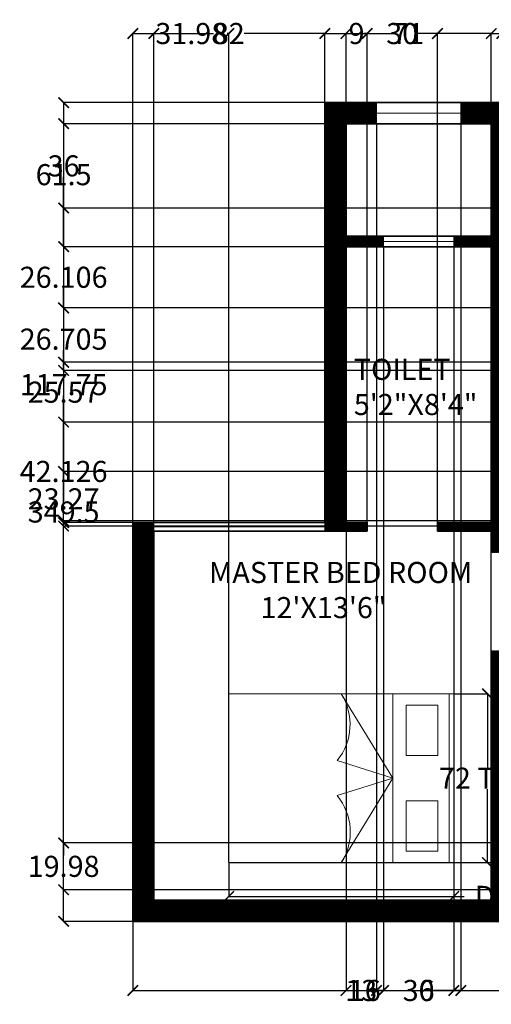
# Model space of a CAD drawing. Units: inches. Extents: x -9 to 675, y 146 to 566.
# Tile 1 of 4: x -9 to 192, y 146 to 566. Entities that reach past the tile are written whole.
import ezdxf

# ---------------------------------------------------------------- set-up
doc = ezdxf.new("R2010")
doc.units = ezdxf.units.IN
doc.header["$MEASUREMENT"] = 0
for name, color, linetype, lineweight in [('A-ANNO-DIMS', 2, 'Continuous', 18), ('A-AREA-IDEN', 7, 'Continuous', 18), ('A-FURN', 8, 'Continuous', 18), ('A-GLAZ', 4, 'Continuous', 18), ('A-WALL', 7, 'Continuous', 35), ('A-WALL-PATT', 252, 'Continuous', 13)]:
    doc.layers.add(name, color=color, linetype=linetype, lineweight=lineweight)
doc.styles.get("Standard").update_dxf_attribs({"font": 'arial.ttf'})
doc.dimstyles.get("Standard").update_dxf_attribs({"dimtxt": 9, "dimasz": 4.5, "dimexe": 0.18, "dimexo": 0.0625, "dimgap": 0.09, "dimtad": 0, "dimtih": 1, "dimtoh": 1, "dimdec": 1, "dimzin": 0, "dimdsep": 46, "dimlunit": 4, "dimtxsty": 'Standard', "dimblk": 'ARCHTICK', "dimcen": 0.09, "dimadec": 0, "dimazin": 0, "dimtfac": 1, "dimtdec": 1, "dimtofl": 0, "dimtmove": 0, "dimatfit": 3, "dimfxl": 1, "dimtolj": 1, "dimtzin": 0, "dimarcsym": 0})

# ---------------------------------------------------------------- blocks, each defined once
blk = doc.blocks.new('BED-DOUBLE-72X96')
for p, q in [((0, 0.1), (0, 72.1)), ((0, 72.1), (96, 72.1)), ((70, 36.1), (48, 72.1)), ((70, 72.1), (70, 0.1)), ((94, 72.1), (94, 0.1)), ((96, 72.1), (96, 0.1)), ((46.29, 43.57), (70, 36.1)), ((70, 36.1), (46.22, 28.65)), ((48, 0.1), (70, 36.1)), ((96, 0.1), (0, 0.1))]:
    blk.add_line(p, q)
for points in [[(89.14, 67.27), (89.14, 45.76), (75.68, 45.76), (75.68, 67.27)], [(89.14, 4.92), (89.14, 26.43), (75.68, 26.43), (75.68, 4.92)]]:
    blk.add_lwpolyline(points, close=True)
for centre, start, end in [((27.13, 59.03), 321.0858, 32.0518), ((27.23, 12.97), 328.2029, 39.5369)]:
    blk.add_arc(centre, 24.62, start, end)
blk = doc.blocks.new('_ArchTick')
at = {"color": 0, "linetype": 'ByBlock', "const_width": 0.15}
blk.add_lwpolyline([(-0.5, -0.5), (0.5, 0.5)], dxfattribs=at)
blk = doc.blocks.new('*D4')
at = {"layer": 'A-ANNO-DIMS', "color": 0, "lineweight": -2, "transparency": 16777216}
for p, q in [((80.28, 206.51), (80.28, 192)), ((176.28, 206.51), (176.28, 192)), ((80.28, 192.18), (176.28, 192.18)), ((176.28, 192.18), (180.78, 192.18))]:
    blk.add_line(p, q, dxfattribs=at)
at = {"layer": 'Defpoints', "color": 0, "transparency": 16777216}
for p in [(80.28, 206.58), (176.28, 206.58), (176.28, 192.18)]:
    blk.add_point(p, dxfattribs=at)
at = {"layer": 'A-ANNO-DIMS', "color": 0, "lineweight": -2, "transparency": 16777216, "xscale": 4.5, "yscale": 4.5, "zscale": 4.5, "rotation": 180}
blk.add_blockref('_ArchTick', (80.28, 192.18), dxfattribs=at)
at = {"layer": 'A-ANNO-DIMS', "color": 0, "lineweight": -2, "transparency": 16777216, "xscale": 4.5, "yscale": 4.5, "zscale": 4.5}
blk.add_blockref('_ArchTick', (176.28, 192.18), dxfattribs=at)
at = {"layer": 'A-ANNO-DIMS', "color": 0, "transparency": 16777216, "insert": (244.83, 192.18), "char_height": 9, "attachment_point": 5}
blk.add_mtext('\\A1;DOUBLE BED 96 TYP.', dxfattribs=at)
blk = doc.blocks.new('*D5')
at = {"layer": 'A-ANNO-DIMS', "color": 0, "lineweight": -2, "transparency": 16777216}
for p, q in [((176.35, 278.67), (190.86, 278.67)), ((190.68, 278.67), (190.68, 247.24)), ((190.68, 206.58), (190.68, 238.01)), ((176.35, 206.58), (190.86, 206.58))]:
    blk.add_line(p, q, dxfattribs=at)
at = {"layer": 'Defpoints', "color": 0, "transparency": 16777216}
for p in [(176.28, 278.67), (190.68, 278.67), (176.28, 206.58)]:
    blk.add_point(p, dxfattribs=at)
at = {"layer": 'A-ANNO-DIMS', "color": 0, "lineweight": -2, "transparency": 16777216, "xscale": 4.5, "yscale": 4.5, "zscale": 4.5}
for p, rotation in [((190.68, 278.67), 90), ((190.68, 206.58), 270)]:
    blk.add_blockref('_ArchTick', p, dxfattribs=dict(at, rotation=rotation))
at = {"layer": 'A-ANNO-DIMS', "color": 0, "transparency": 16777216, "insert": (190.68, 242.63), "char_height": 9, "attachment_point": 5}
blk.add_mtext('\\A1;72 TYP.', dxfattribs=at)
blk = doc.blocks.new('*D8')
at = {"layer": 'A-ANNO-DIMS', "color": 0, "lineweight": -2, "transparency": 16777216}
for p, q in [((626.3, 217.45), (626.3, 151.83)), ((39.3, 181.45), (39.3, 151.83)), ((39.3, 152.01), (322.77, 152.01)), ((626.3, 152.01), (342.83, 152.01))]:
    blk.add_line(p, q, dxfattribs=at)
at = {"layer": 'Defpoints', "color": 0, "transparency": 16777216}
for p in [(626.3, 217.51), (39.3, 181.51), (626.3, 152.01)]:
    blk.add_point(p, dxfattribs=at)
at = {"layer": 'A-ANNO-DIMS', "color": 0, "lineweight": -2, "transparency": 16777216, "xscale": 4.5, "yscale": 4.5, "zscale": 4.5, "rotation": 180}
blk.add_blockref('_ArchTick', (39.3, 152.01), dxfattribs=at)
at = {"layer": 'A-ANNO-DIMS', "color": 0, "lineweight": -2, "transparency": 16777216, "xscale": 4.5, "yscale": 4.5, "zscale": 4.5}
blk.add_blockref('_ArchTick', (626.3, 152.01), dxfattribs=at)
at = {"layer": 'A-ANNO-DIMS', "color": 0, "transparency": 16777216, "insert": (332.8, 152.01), "char_height": 9, "attachment_point": 5}
blk.add_mtext('\\A1;587', dxfattribs=at)
blk = doc.blocks.new('*D9')
at = {"layer": 'A-ANNO-DIMS', "color": 0, "lineweight": -2, "transparency": 16777216}
for p, q in [((121.24, 531.01), (9.62, 531.01)), ((9.8, 531.01), (9.8, 360.95)), ((9.8, 181.51), (9.8, 351.57)), ((39.24, 181.51), (9.62, 181.51))]:
    blk.add_line(p, q, dxfattribs=at)
at = {"layer": 'Defpoints', "color": 0, "transparency": 16777216}
for p in [(9.8, 531.01), (121.3, 531.01), (39.3, 181.51)]:
    blk.add_point(p, dxfattribs=at)
at = {"layer": 'A-ANNO-DIMS', "color": 0, "lineweight": -2, "transparency": 16777216, "xscale": 4.5, "yscale": 4.5, "zscale": 4.5}
for p, rotation in [((9.8, 531.01), 90), ((9.8, 181.51), 270)]:
    blk.add_blockref('_ArchTick', p, dxfattribs=dict(at, rotation=rotation))
at = {"layer": 'A-ANNO-DIMS', "color": 0, "transparency": 16777216, "insert": (9.8, 356.26), "char_height": 9, "attachment_point": 5}
blk.add_mtext('\\A1;349.5', dxfattribs=at)
blk = doc.blocks.new('*D10')
at = {"layer": 'A-ANNO-DIMS', "color": 0, "lineweight": -2, "transparency": 16777216}
for p, q in [((39.3, 351.82), (39.3, 560.69)), ((39.3, 560.51), (73.81, 560.51)), ((121.3, 560.51), (86.8, 560.51)), ((121.3, 351.82), (121.3, 560.69))]:
    blk.add_line(p, q, dxfattribs=at)
at = {"layer": 'Defpoints', "color": 0, "transparency": 16777216}
for p in [(121.3, 560.51), (39.3, 351.76), (121.3, 351.76)]:
    blk.add_point(p, dxfattribs=at)
at = {"layer": 'A-ANNO-DIMS', "color": 0, "lineweight": -2, "transparency": 16777216, "xscale": 4.5, "yscale": 4.5, "zscale": 4.5, "rotation": 180}
blk.add_blockref('_ArchTick', (39.3, 560.51), dxfattribs=at)
at = {"layer": 'A-ANNO-DIMS', "color": 0, "lineweight": -2, "transparency": 16777216, "xscale": 4.5, "yscale": 4.5, "zscale": 4.5}
blk.add_blockref('_ArchTick', (121.3, 560.51), dxfattribs=at)
at = {"layer": 'A-ANNO-DIMS', "color": 0, "transparency": 16777216, "insert": (80.3, 560.51), "char_height": 9, "attachment_point": 5}
blk.add_mtext('\\A1;82', dxfattribs=at)
blk = doc.blocks.new('*D11')
at = {"layer": 'A-ANNO-DIMS', "color": 0, "lineweight": -2, "transparency": 16777216}
for p, q in [((121.3, 531.07), (121.3, 560.69)), ((121.3, 560.51), (151.17, 560.51)), ((192.3, 560.51), (162.43, 560.51)), ((192.3, 522.07), (192.3, 560.69))]:
    blk.add_line(p, q, dxfattribs=at)
at = {"layer": 'Defpoints', "color": 0, "transparency": 16777216}
for p in [(192.3, 560.51), (121.3, 531.01), (192.3, 522.01)]:
    blk.add_point(p, dxfattribs=at)
at = {"layer": 'A-ANNO-DIMS', "color": 0, "lineweight": -2, "transparency": 16777216, "xscale": 4.5, "yscale": 4.5, "zscale": 4.5, "rotation": 180}
blk.add_blockref('_ArchTick', (121.3, 560.51), dxfattribs=at)
at = {"layer": 'A-ANNO-DIMS', "color": 0, "lineweight": -2, "transparency": 16777216, "xscale": 4.5, "yscale": 4.5, "zscale": 4.5}
blk.add_blockref('_ArchTick', (192.3, 560.51), dxfattribs=at)
at = {"layer": 'A-ANNO-DIMS', "color": 0, "transparency": 16777216, "insert": (156.8, 560.51), "char_height": 9, "attachment_point": 5}
blk.add_mtext('\\A1;71', dxfattribs=at)
blk = doc.blocks.new('*D12')
at = {"layer": 'A-ANNO-DIMS', "color": 0, "lineweight": -2, "transparency": 16777216}
for p, q in [((192.3, 522.07), (192.3, 560.69)), ((192.3, 560.51), (227.74, 560.51)), ((286.8, 560.51), (251.37, 560.51)), ((286.8, 531.07), (286.8, 560.69))]:
    blk.add_line(p, q, dxfattribs=at)
at = {"layer": 'Defpoints', "color": 0, "transparency": 16777216}
for p in [(286.8, 560.51), (286.8, 531.01), (192.3, 522.01)]:
    blk.add_point(p, dxfattribs=at)
at = {"layer": 'A-ANNO-DIMS', "color": 0, "lineweight": -2, "transparency": 16777216, "xscale": 4.5, "yscale": 4.5, "zscale": 4.5, "rotation": 180}
blk.add_blockref('_ArchTick', (192.3, 560.51), dxfattribs=at)
at = {"layer": 'A-ANNO-DIMS', "color": 0, "lineweight": -2, "transparency": 16777216, "xscale": 4.5, "yscale": 4.5, "zscale": 4.5}
blk.add_blockref('_ArchTick', (286.8, 560.51), dxfattribs=at)
at = {"layer": 'A-ANNO-DIMS', "color": 0, "transparency": 16777216, "insert": (239.55, 560.51), "char_height": 9, "attachment_point": 5}
blk.add_mtext('\\A1;94.5', dxfattribs=at)
blk = doc.blocks.new('*D16')
at = {"layer": 'A-ANNO-DIMS', "color": 0, "lineweight": -2, "transparency": 16777216}
for p, q in [((130.24, 469.51), (9.62, 469.51)), ((9.8, 469.51), (9.8, 415.32)), ((9.8, 351.76), (9.8, 405.95)), ((121.24, 351.76), (9.62, 351.76))]:
    blk.add_line(p, q, dxfattribs=at)
at = {"layer": 'Defpoints', "color": 0, "transparency": 16777216}
for p in [(9.8, 469.51), (130.3, 469.51), (121.3, 351.76)]:
    blk.add_point(p, dxfattribs=at)
at = {"layer": 'A-ANNO-DIMS', "color": 0, "lineweight": -2, "transparency": 16777216, "xscale": 4.5, "yscale": 4.5, "zscale": 4.5}
for p, rotation in [((9.8, 469.51), 90), ((9.8, 351.76), 270)]:
    blk.add_blockref('_ArchTick', p, dxfattribs=dict(at, rotation=rotation))
at = {"layer": 'A-ANNO-DIMS', "color": 0, "transparency": 16777216, "insert": (9.8, 410.63), "char_height": 9, "attachment_point": 5}
blk.add_mtext('\\A1;117.75', dxfattribs=at)
blk = doc.blocks.new('*D17')
at = {"layer": 'A-ANNO-DIMS', "color": 0, "lineweight": -2, "transparency": 16777216}
for p, q in [((121.24, 531.01), (9.62, 531.01)), ((9.8, 531.01), (9.8, 504.94)), ((9.8, 469.51), (9.8, 495.57)), ((130.24, 469.51), (9.62, 469.51))]:
    blk.add_line(p, q, dxfattribs=at)
at = {"layer": 'Defpoints', "color": 0, "transparency": 16777216}
for p in [(9.8, 531.01), (121.3, 531.01), (130.3, 469.51)]:
    blk.add_point(p, dxfattribs=at)
at = {"layer": 'A-ANNO-DIMS', "color": 0, "lineweight": -2, "transparency": 16777216, "xscale": 4.5, "yscale": 4.5, "zscale": 4.5}
for p, rotation in [((9.8, 531.01), 90), ((9.8, 469.51), 270)]:
    blk.add_blockref('_ArchTick', p, dxfattribs=dict(at, rotation=rotation))
at = {"layer": 'A-ANNO-DIMS', "color": 0, "transparency": 16777216, "insert": (9.8, 500.26), "char_height": 9, "attachment_point": 5}
blk.add_mtext('\\A1;61.5', dxfattribs=at)
blk = doc.blocks.new('*D24')
at = {"layer": 'A-ANNO-DIMS', "color": 0, "lineweight": -2, "transparency": 16777216}
for p, q in [((130.3, 521.95), (130.3, 151.83)), ((143.3, 521.95), (143.3, 151.83)), ((130.3, 152.01), (130.69, 152.01)), ((143.3, 152.01), (142.92, 152.01))]:
    blk.add_line(p, q, dxfattribs=at)
at = {"layer": 'Defpoints', "color": 0, "transparency": 16777216}
for p in [(130.3, 522.01), (143.3, 522.01), (143.3, 152.01)]:
    blk.add_point(p, dxfattribs=at)
at = {"layer": 'A-ANNO-DIMS', "color": 0, "lineweight": -2, "transparency": 16777216, "xscale": 4.5, "yscale": 4.5, "zscale": 4.5, "rotation": 180}
blk.add_blockref('_ArchTick', (130.3, 152.01), dxfattribs=at)
at = {"layer": 'A-ANNO-DIMS', "color": 0, "lineweight": -2, "transparency": 16777216, "xscale": 4.5, "yscale": 4.5, "zscale": 4.5}
blk.add_blockref('_ArchTick', (143.3, 152.01), dxfattribs=at)
at = {"layer": 'A-ANNO-DIMS', "color": 0, "transparency": 16777216, "insert": (136.8, 152.01), "char_height": 9, "attachment_point": 5}
blk.add_mtext('\\A1;13', dxfattribs=at)
blk = doc.blocks.new('*D25')
at = {"layer": 'A-ANNO-DIMS', "color": 0, "lineweight": -2, "transparency": 16777216}
for p, q in [((143.3, 521.95), (143.3, 151.83)), ((179.3, 521.95), (179.3, 151.83)), ((143.3, 152.01), (154.77, 152.01)), ((179.3, 152.01), (167.83, 152.01))]:
    blk.add_line(p, q, dxfattribs=at)
at = {"layer": 'Defpoints', "color": 0, "transparency": 16777216}
for p in [(143.3, 522.01), (179.3, 522.01), (179.3, 152.01)]:
    blk.add_point(p, dxfattribs=at)
at = {"layer": 'A-ANNO-DIMS', "color": 0, "lineweight": -2, "transparency": 16777216, "xscale": 4.5, "yscale": 4.5, "zscale": 4.5, "rotation": 180}
blk.add_blockref('_ArchTick', (143.3, 152.01), dxfattribs=at)
at = {"layer": 'A-ANNO-DIMS', "color": 0, "lineweight": -2, "transparency": 16777216, "xscale": 4.5, "yscale": 4.5, "zscale": 4.5}
blk.add_blockref('_ArchTick', (179.3, 152.01), dxfattribs=at)
at = {"layer": 'A-ANNO-DIMS', "color": 0, "transparency": 16777216, "insert": (161.3, 152.01), "char_height": 9, "attachment_point": 5}
blk.add_mtext('\\A1;36', dxfattribs=at)
blk = doc.blocks.new('*D31')
at = {"layer": 'A-ANNO-DIMS', "color": 0, "lineweight": -2, "transparency": 16777216}
for p, q in [((130.3, 351.82), (130.3, 560.69)), ((130.3, 560.51), (131.75, 560.51)), ((139.3, 560.51), (137.85, 560.51)), ((139.3, 351.82), (139.3, 560.69))]:
    blk.add_line(p, q, dxfattribs=at)
at = {"layer": 'Defpoints', "color": 0, "transparency": 16777216}
for p in [(139.3, 560.51), (130.3, 351.76), (139.3, 351.76)]:
    blk.add_point(p, dxfattribs=at)
at = {"layer": 'A-ANNO-DIMS', "color": 0, "lineweight": -2, "transparency": 16777216, "xscale": 4.5, "yscale": 4.5, "zscale": 4.5, "rotation": 180}
blk.add_blockref('_ArchTick', (130.3, 560.51), dxfattribs=at)
at = {"layer": 'A-ANNO-DIMS', "color": 0, "lineweight": -2, "transparency": 16777216, "xscale": 4.5, "yscale": 4.5, "zscale": 4.5}
blk.add_blockref('_ArchTick', (139.3, 560.51), dxfattribs=at)
at = {"layer": 'A-ANNO-DIMS', "color": 0, "transparency": 16777216, "insert": (134.8, 560.51), "char_height": 9, "attachment_point": 5}
blk.add_mtext('\\A1;9', dxfattribs=at)
blk = doc.blocks.new('*D32')
at = {"layer": 'A-ANNO-DIMS', "color": 0, "lineweight": -2, "transparency": 16777216}
for p, q in [((139.3, 351.82), (139.3, 560.69)), ((139.3, 560.51), (147.78, 560.51)), ((169.3, 560.51), (160.82, 560.51)), ((169.3, 351.82), (169.3, 560.69))]:
    blk.add_line(p, q, dxfattribs=at)
at = {"layer": 'Defpoints', "color": 0, "transparency": 16777216}
for p in [(169.3, 560.51), (139.3, 351.76), (169.3, 351.76)]:
    blk.add_point(p, dxfattribs=at)
at = {"layer": 'A-ANNO-DIMS', "color": 0, "lineweight": -2, "transparency": 16777216, "xscale": 4.5, "yscale": 4.5, "zscale": 4.5, "rotation": 180}
blk.add_blockref('_ArchTick', (139.3, 560.51), dxfattribs=at)
at = {"layer": 'A-ANNO-DIMS', "color": 0, "lineweight": -2, "transparency": 16777216, "xscale": 4.5, "yscale": 4.5, "zscale": 4.5}
blk.add_blockref('_ArchTick', (169.3, 560.51), dxfattribs=at)
at = {"layer": 'A-ANNO-DIMS', "color": 0, "transparency": 16777216, "insert": (154.3, 560.51), "char_height": 9, "attachment_point": 5}
blk.add_mtext('\\A1;30', dxfattribs=at)
blk = doc.blocks.new('*D39')
at = {"layer": 'A-ANNO-DIMS', "color": 0, "lineweight": -2, "transparency": 16777216}
for p, q in [((357.24, 214.99), (9.62, 214.99)), ((9.8, 214.99), (9.8, 209.69)), ((9.8, 195.01), (9.8, 200.32)), ((357.24, 195.01), (9.62, 195.01))]:
    blk.add_line(p, q, dxfattribs=at)
at = {"layer": 'Defpoints', "color": 0, "transparency": 16777216}
for p in [(9.8, 214.99), (357.3, 214.99), (357.3, 195.01)]:
    blk.add_point(p, dxfattribs=at)
at = {"layer": 'A-ANNO-DIMS', "color": 0, "lineweight": -2, "transparency": 16777216, "xscale": 4.5, "yscale": 4.5, "zscale": 4.5}
for p, rotation in [((9.8, 214.99), 90), ((9.8, 195.01), 270)]:
    blk.add_blockref('_ArchTick', p, dxfattribs=dict(at, rotation=rotation))
at = {"layer": 'A-ANNO-DIMS', "color": 0, "transparency": 16777216, "insert": (9.8, 205), "char_height": 9, "attachment_point": 5}
blk.add_mtext('\\A1;19.98', dxfattribs=at)
blk = doc.blocks.new('*D40')
at = {"layer": 'A-ANNO-DIMS', "color": 0, "lineweight": -2, "transparency": 16777216}
for p, q in [((146.3, 469.45), (146.3, 151.83)), ((176.3, 469.45), (176.3, 151.83)), ((146.3, 152.01), (154.78, 152.01)), ((176.3, 152.01), (167.82, 152.01))]:
    blk.add_line(p, q, dxfattribs=at)
at = {"layer": 'Defpoints', "color": 0, "transparency": 16777216}
for p in [(146.3, 469.51), (176.3, 469.51), (176.3, 152.01)]:
    blk.add_point(p, dxfattribs=at)
at = {"layer": 'A-ANNO-DIMS', "color": 0, "lineweight": -2, "transparency": 16777216, "xscale": 4.5, "yscale": 4.5, "zscale": 4.5, "rotation": 180}
blk.add_blockref('_ArchTick', (146.3, 152.01), dxfattribs=at)
at = {"layer": 'A-ANNO-DIMS', "color": 0, "lineweight": -2, "transparency": 16777216, "xscale": 4.5, "yscale": 4.5, "zscale": 4.5}
blk.add_blockref('_ArchTick', (176.3, 152.01), dxfattribs=at)
at = {"layer": 'A-ANNO-DIMS', "color": 0, "transparency": 16777216, "insert": (161.3, 152.01), "char_height": 9, "attachment_point": 5}
blk.add_mtext('\\A1;30', dxfattribs=at)
blk = doc.blocks.new('*D41')
at = {"layer": 'A-ANNO-DIMS', "color": 0, "lineweight": -2, "transparency": 16777216}
for p, q in [((130.3, 469.45), (130.3, 151.83)), ((146.3, 469.45), (146.3, 151.83)), ((130.3, 152.01), (132.19, 152.01)), ((146.3, 152.01), (144.41, 152.01))]:
    blk.add_line(p, q, dxfattribs=at)
at = {"layer": 'Defpoints', "color": 0, "transparency": 16777216}
for p in [(130.3, 469.51), (146.3, 469.51), (146.3, 152.01)]:
    blk.add_point(p, dxfattribs=at)
at = {"layer": 'A-ANNO-DIMS', "color": 0, "lineweight": -2, "transparency": 16777216, "xscale": 4.5, "yscale": 4.5, "zscale": 4.5, "rotation": 180}
blk.add_blockref('_ArchTick', (130.3, 152.01), dxfattribs=at)
at = {"layer": 'A-ANNO-DIMS', "color": 0, "lineweight": -2, "transparency": 16777216, "xscale": 4.5, "yscale": 4.5, "zscale": 4.5}
blk.add_blockref('_ArchTick', (146.3, 152.01), dxfattribs=at)
at = {"layer": 'A-ANNO-DIMS', "color": 0, "transparency": 16777216, "insert": (138.3, 152.01), "char_height": 9, "attachment_point": 5}
blk.add_mtext('\\A1;16', dxfattribs=at)
blk = doc.blocks.new('*D44')
at = {"layer": 'A-ANNO-DIMS', "color": 0, "lineweight": -2, "transparency": 16777216}
for p, q in [((48.3, 190.57), (48.3, 560.69)), ((48.3, 560.51), (49.01, 560.51)), ((80.28, 560.51), (79.57, 560.51)), ((80.28, 206.74), (80.28, 560.69))]:
    blk.add_line(p, q, dxfattribs=at)
at = {"layer": 'Defpoints', "color": 0, "transparency": 16777216}
for p in [(80.28, 560.51), (80.28, 206.67), (48.3, 190.51)]:
    blk.add_point(p, dxfattribs=at)
at = {"layer": 'A-ANNO-DIMS', "color": 0, "lineweight": -2, "transparency": 16777216, "xscale": 4.5, "yscale": 4.5, "zscale": 4.5, "rotation": 180}
blk.add_blockref('_ArchTick', (48.3, 560.51), dxfattribs=at)
at = {"layer": 'A-ANNO-DIMS', "color": 0, "lineweight": -2, "transparency": 16777216, "xscale": 4.5, "yscale": 4.5, "zscale": 4.5}
blk.add_blockref('_ArchTick', (80.28, 560.51), dxfattribs=at)
at = {"layer": 'A-ANNO-DIMS', "color": 0, "transparency": 16777216, "insert": (64.29, 560.51), "char_height": 9, "attachment_point": 5}
blk.add_mtext('\\A1;31.98', dxfattribs=at)
blk = doc.blocks.new('*D45')
at = {"layer": 'A-ANNO-DIMS', "color": 0, "lineweight": -2, "transparency": 16777216}
for p, q in [((80.35, 206.67), (655.98, 206.67)), ((655.8, 206.67), (655.8, 203.28)), ((655.8, 190.51), (655.8, 193.91)), ((48.37, 190.51), (655.98, 190.51))]:
    blk.add_line(p, q, dxfattribs=at)
at = {"layer": 'Defpoints', "color": 0, "transparency": 16777216}
for p in [(80.28, 206.67), (655.8, 206.67), (48.3, 190.51)]:
    blk.add_point(p, dxfattribs=at)
at = {"layer": 'A-ANNO-DIMS', "color": 0, "lineweight": -2, "transparency": 16777216, "xscale": 4.5, "yscale": 4.5, "zscale": 4.5}
for p, rotation in [((655.8, 206.67), 90), ((655.8, 190.51), 270)]:
    blk.add_blockref('_ArchTick', p, dxfattribs=dict(at, rotation=rotation))
at = {"layer": 'A-ANNO-DIMS', "color": 0, "transparency": 16777216, "insert": (655.8, 198.59), "char_height": 9, "attachment_point": 5}
blk.add_mtext('\\A1;16.165', dxfattribs=at)
blk = doc.blocks.new('*D46')
at = {"layer": 'A-ANNO-DIMS', "color": 0, "lineweight": -2, "transparency": 16777216}
for p, q in [((435.74, 522.01), (9.62, 522.01)), ((9.8, 522.01), (9.8, 508.7)), ((9.8, 486.01), (9.8, 499.32)), ((445.74, 486.01), (9.62, 486.01))]:
    blk.add_line(p, q, dxfattribs=at)
at = {"layer": 'Defpoints', "color": 0, "transparency": 16777216}
for p in [(435.8, 522.01), (9.8, 486.01), (445.8, 486.01)]:
    blk.add_point(p, dxfattribs=at)
at = {"layer": 'A-ANNO-DIMS', "color": 0, "lineweight": -2, "transparency": 16777216, "xscale": 4.5, "yscale": 4.5, "zscale": 4.5}
for p, rotation in [((9.8, 522.01), 90), ((9.8, 486.01), 270)]:
    blk.add_blockref('_ArchTick', p, dxfattribs=dict(at, rotation=rotation))
at = {"layer": 'A-ANNO-DIMS', "color": 0, "transparency": 16777216, "insert": (9.8, 504.01), "char_height": 9, "attachment_point": 5}
blk.add_mtext('\\A1;36', dxfattribs=at)
blk = doc.blocks.new('*D47')
at = {"layer": 'A-ANNO-DIMS', "color": 0, "lineweight": -2, "transparency": 16777216}
for p, q in [((617.24, 373.51), (9.62, 373.51)), ((9.8, 373.51), (9.8, 366.56)), ((9.8, 350.24), (9.8, 357.19)), ((602.52, 350.24), (9.62, 350.24))]:
    blk.add_line(p, q, dxfattribs=at)
at = {"layer": 'Defpoints', "color": 0, "transparency": 16777216}
for p in [(617.3, 373.51), (9.8, 350.24), (602.59, 350.24)]:
    blk.add_point(p, dxfattribs=at)
at = {"layer": 'A-ANNO-DIMS', "color": 0, "lineweight": -2, "transparency": 16777216, "xscale": 4.5, "yscale": 4.5, "zscale": 4.5}
for p, rotation in [((9.8, 373.51), 90), ((9.8, 350.24), 270)]:
    blk.add_blockref('_ArchTick', p, dxfattribs=dict(at, rotation=rotation))
at = {"layer": 'A-ANNO-DIMS', "color": 0, "transparency": 16777216, "insert": (9.8, 361.87), "char_height": 9, "attachment_point": 5}
blk.add_mtext('\\A1;23.27', dxfattribs=at)
blk = doc.blocks.new('*D50')
at = {"layer": 'A-ANNO-DIMS', "color": 0, "lineweight": -2, "transparency": 16777216}
for p, q in [((192.3, 297.07), (192.3, 560.69)), ((192.3, 560.51), (196.8, 560.51)), ((196.8, 297.07), (196.8, 560.69)), ((196.8, 560.51), (201.3, 560.51))]:
    blk.add_line(p, q, dxfattribs=at)
at = {"layer": 'Defpoints', "color": 0, "transparency": 16777216}
for p in [(196.8, 560.51), (192.3, 297.01), (196.8, 297.01)]:
    blk.add_point(p, dxfattribs=at)
at = {"layer": 'A-ANNO-DIMS', "color": 0, "lineweight": -2, "transparency": 16777216, "xscale": 4.5, "yscale": 4.5, "zscale": 4.5, "rotation": 180}
blk.add_blockref('_ArchTick', (192.3, 560.51), dxfattribs=at)
at = {"layer": 'A-ANNO-DIMS', "color": 0, "lineweight": -2, "transparency": 16777216, "xscale": 4.5, "yscale": 4.5, "zscale": 4.5}
blk.add_blockref('_ArchTick', (196.8, 560.51), dxfattribs=at)
at = {"layer": 'A-ANNO-DIMS', "color": 0, "transparency": 16777216, "insert": (209.8, 560.51), "char_height": 9, "attachment_point": 5}
blk.add_mtext('\\A1;4.5', dxfattribs=at)
blk = doc.blocks.new('*D52')
at = {"layer": 'A-ANNO-DIMS', "color": 0, "lineweight": -2, "transparency": 16777216}
for p, q in [((266.3, 443.4), (9.62, 443.4)), ((9.8, 443.4), (9.8, 434.74)), ((9.8, 416.7), (9.8, 425.37)), ((266.3, 416.7), (9.62, 416.7))]:
    blk.add_line(p, q, dxfattribs=at)
at = {"layer": 'Defpoints', "color": 0, "transparency": 16777216}
for p in [(9.8, 443.4), (266.36, 443.4), (266.36, 416.7)]:
    blk.add_point(p, dxfattribs=at)
at = {"layer": 'A-ANNO-DIMS', "color": 0, "lineweight": -2, "transparency": 16777216, "xscale": 4.5, "yscale": 4.5, "zscale": 4.5}
for p, rotation in [((9.8, 443.4), 90), ((9.8, 416.7), 270)]:
    blk.add_blockref('_ArchTick', p, dxfattribs=dict(at, rotation=rotation))
at = {"layer": 'A-ANNO-DIMS', "color": 0, "transparency": 16777216, "insert": (9.8, 430.05), "char_height": 9, "attachment_point": 5}
blk.add_mtext('\\A1;26.705', dxfattribs=at)
blk = doc.blocks.new('*D53')
at = {"layer": 'A-ANNO-DIMS', "color": 0, "lineweight": -2, "transparency": 16777216}
for p, q in [((261.31, 469.51), (9.62, 469.51)), ((9.8, 469.51), (9.8, 461.14)), ((9.8, 443.4), (9.8, 451.77)), ((266.3, 443.4), (9.62, 443.4))]:
    blk.add_line(p, q, dxfattribs=at)
at = {"layer": 'Defpoints', "color": 0, "transparency": 16777216}
for p in [(261.37, 469.51), (9.8, 443.4), (266.36, 443.4)]:
    blk.add_point(p, dxfattribs=at)
at = {"layer": 'A-ANNO-DIMS', "color": 0, "lineweight": -2, "transparency": 16777216, "xscale": 4.5, "yscale": 4.5, "zscale": 4.5}
for p, rotation in [((9.8, 469.51), 90), ((9.8, 443.4), 270)]:
    blk.add_blockref('_ArchTick', p, dxfattribs=dict(at, rotation=rotation))
at = {"layer": 'A-ANNO-DIMS', "color": 0, "transparency": 16777216, "insert": (9.8, 456.46), "char_height": 9, "attachment_point": 5}
blk.add_mtext('\\A1;26.106', dxfattribs=at)
blk = doc.blocks.new('*D55')
at = {"layer": 'A-ANNO-DIMS', "color": 0, "lineweight": -2, "transparency": 16777216}
for p, q in [((202.15, 420.2), (9.62, 420.2)), ((9.8, 420.2), (9.8, 412.11)), ((9.8, 394.64), (9.8, 402.74)), ((202.15, 394.64), (9.62, 394.64))]:
    blk.add_line(p, q, dxfattribs=at)
at = {"layer": 'Defpoints', "color": 0, "transparency": 16777216}
for p in [(9.8, 420.2), (202.21, 420.2), (202.21, 394.64)]:
    blk.add_point(p, dxfattribs=at)
at = {"layer": 'A-ANNO-DIMS', "color": 0, "lineweight": -2, "transparency": 16777216, "xscale": 4.5, "yscale": 4.5, "zscale": 4.5}
for p, rotation in [((9.8, 420.2), 90), ((9.8, 394.64), 270)]:
    blk.add_blockref('_ArchTick', p, dxfattribs=dict(at, rotation=rotation))
at = {"layer": 'A-ANNO-DIMS', "color": 0, "transparency": 16777216, "insert": (9.8, 407.42), "char_height": 9, "attachment_point": 5}
blk.add_mtext('\\A1;25.57', dxfattribs=at)
blk = doc.blocks.new('*D56')
at = {"layer": 'A-ANNO-DIMS', "color": 0, "lineweight": -2, "transparency": 16777216}
for p, q in [((202.15, 394.64), (9.62, 394.64)), ((9.8, 394.64), (9.8, 378.26)), ((9.8, 352.51), (9.8, 368.89)), ((196.74, 352.51), (9.62, 352.51))]:
    blk.add_line(p, q, dxfattribs=at)
at = {"layer": 'Defpoints', "color": 0, "transparency": 16777216}
for p in [(9.8, 394.64), (202.21, 394.64), (196.8, 352.51)]:
    blk.add_point(p, dxfattribs=at)
at = {"layer": 'A-ANNO-DIMS', "color": 0, "lineweight": -2, "transparency": 16777216, "xscale": 4.5, "yscale": 4.5, "zscale": 4.5}
for p, rotation in [((9.8, 394.64), 90), ((9.8, 352.51), 270)]:
    blk.add_blockref('_ArchTick', p, dxfattribs=dict(at, rotation=rotation))
at = {"layer": 'A-ANNO-DIMS', "color": 0, "transparency": 16777216, "insert": (9.8, 373.57), "char_height": 9, "attachment_point": 5}
blk.add_mtext('\\A1;42.126', dxfattribs=at)

msp = doc.modelspace()

# ---------------------------------------------------------------- hatches: boundary and pattern name
at = {"layer": 'A-WALL-PATT'}
h = msp.add_hatch(dxfattribs=at)
h.set_pattern_fill('ANSI31', color=256)
h.paths.add_polyline_path([(361.8026, 244.5097), (357.3026, 244.5097), (357.3026, 228.4917), (286.8026, 228.4917), (196.8026, 228.4917), (196.8026, 297.0097), (192.3026, 297.0097), (192.3026, 190.5097), (196.8026, 190.5097), (196.8026, 219.4917), (286.8026, 219.4917), (357.3026, 219.4917), (357.3026, 217.5097), (357.3026, 214.9917), (361.8026, 214.9917), (361.8026, 217.5097)])
h.paths.add_polyline_path([(532.6092, 217.5097), (541.8026, 217.5097), (550.8026, 217.5097), (626.3026, 217.5097), (626.3026, 373.5097), (626.3026, 378.0097), (617.3026, 378.0097), (617.3026, 373.5097), (617.3026, 226.5097), (550.8026, 226.5097), (541.8026, 226.5097), (488.3026, 226.5097), (488.3026, 331.0097), (483.8026, 331.0097), (474.8026, 331.0097), (474.8026, 326.5097), (483.8026, 326.5097), (483.8026, 226.5097), (421.8026, 226.5097), (421.8026, 326.5097), (444.8026, 326.5097), (444.8026, 331.0097), (421.8026, 331.0097), (417.3026, 331.0097), (417.3026, 217.5097), (417.3026, 190.5097), (387.6027, 190.5097), (361.8026, 190.5097), (361.8026, 195.0097), (357.3026, 195.0097), (357.3026, 190.5097), (357.3026, 181.5097), (387.6027, 181.5097), (421.8026, 181.5097), (532.6092, 181.5097)])
h.paths.add_polyline_path([(421.8026, 190.5097), (421.8026, 217.5097), (523.6092, 217.5097), (523.6092, 190.5097)], flags=16)
h.paths.add_polyline_path([(550.8026, 378.0097), (550.8026, 531.0097), (525.3955, 531.0097), (525.3955, 522.0097), (541.8026, 522.0097), (541.8026, 378.0097), (472.8026, 378.0097), (472.8026, 373.5097), (483.8026, 373.5097), (488.3026, 373.5097), (541.8026, 373.5097), (550.8026, 373.5097)])
h.paths.add_polyline_path([(130.3026, 469.5097), (146.3026, 469.5097), (146.3026, 474.0097), (130.3026, 474.0097), (130.3026, 522.0097), (143.3026, 522.0097), (143.3026, 531.0097), (121.3026, 531.0097), (121.3026, 351.7597), (121.3026, 348.0097), (130.3026, 348.0097), (139.3026, 348.0097), (139.3026, 351.7597), (130.3026, 351.7597)])
h.paths.add_polyline_path([(211.9624, 531.0097), (179.3026, 531.0097), (179.3026, 522.0097), (192.3026, 522.0097), (192.3026, 474.0097), (176.3026, 474.0097), (176.3026, 469.5097), (192.3026, 469.5097), (192.3026, 351.7597), (169.3026, 351.7597), (169.3026, 348.0097), (192.3026, 348.0097), (192.3026, 339.0097), (196.8026, 339.0097), (196.8026, 348.0097), (226.8026, 348.0097), (226.8026, 352.5097), (196.8026, 352.5097), (196.8026, 469.5097), (226.8026, 469.5097), (226.8026, 474.0097), (196.8026, 474.0097), (196.8026, 522.0097), (211.9624, 522.0097)])
h.paths.add_polyline_path([(291.3026, 522.0097), (291.3026, 531.0097), (286.8026, 531.0097), (286.8026, 522.0097), (286.8026, 352.5097), (256.8026, 352.5097), (256.8026, 348.0097), (286.8026, 348.0097), (286.8026, 346.5097), (291.3026, 346.5097)])
h.paths.add_polyline_path([(417.3026, 474.0097), (291.3026, 474.0097), (291.3026, 469.5097), (417.3026, 469.5097)])
h.paths.add_polyline_path([(421.8026, 522.0097), (435.8002, 522.0097), (435.8002, 531.0097), (417.3026, 531.0097), (417.3026, 522.0097), (417.3026, 373.5097), (421.8026, 373.5097), (430.8026, 373.5097), (430.8026, 378.0097), (421.8026, 378.0097)])
h.paths.add_polyline_path([(48.3026, 348.0097), (48.3026, 351.7597), (39.3026, 351.7597), (39.3026, 348.0097), (39.3026, 181.5097), (121.3026, 181.5097), (196.8026, 181.5097), (196.8026, 190.5097), (192.3026, 190.5097), (121.3026, 190.5097), (48.3026, 190.5097)])

# ---------------------------------------------------------------- linework, layer by layer
at = {"layer": 'A-GLAZ'}
for p, q in [((143.3026, 531.0097), (143.3026, 522.0097)), ((179.3026, 531.0097), (179.3026, 522.0097)), ((143.3026, 526.5097), (179.3026, 526.5097)), ((146.3026, 474.0097), (146.3026, 469.5097)), ((146.3026, 471.7597), (176.3026, 471.7597)), ((176.3026, 474.0097), (176.3026, 469.5097)), ((48.3026, 348.0097), (48.3026, 351.7597)), ((48.3026, 349.8847), (121.3026, 349.8847)), ((121.3026, 351.7597), (121.3026, 348.0097))]:
    msp.add_line(p, q, dxfattribs=at)
at = {"layer": 'A-WALL'}
for p, q in [((121.3026, 531.0097), (121.3026, 351.7597)), ((121.3026, 531.0097), (550.8026, 531.0097)), ((130.3026, 522.0097), (130.3026, 474.0097)), ((130.3026, 522.0097), (192.3026, 522.0097)), ((192.3026, 522.0097), (192.3026, 474.0097)), ((192.3026, 474.0097), (130.3026, 474.0097)), ((192.3026, 469.5097), (130.3026, 469.5097)), ((130.3026, 469.5097), (130.3026, 351.7597)), ((192.3026, 469.5097), (192.3026, 351.7597)), ((121.3026, 351.7597), (39.3026, 351.7597)), ((39.3026, 348.0097), (39.3026, 351.7597)), ((139.3026, 351.7597), (130.3026, 351.7597)), ((139.3026, 351.7597), (139.3026, 348.0097)), ((192.3026, 351.7597), (169.3026, 351.7597)), ((169.3026, 351.7597), (169.3026, 348.0097)), ((39.3026, 348.0097), (39.3026, 181.5097)), ((48.3026, 348.0097), (48.3026, 190.5097)), ((130.3026, 348.0097), (48.3026, 348.0097)), ((139.3026, 348.0097), (130.3026, 348.0097)), ((192.3026, 348.0097), (169.3026, 348.0097)), ((192.3026, 348.0097), (192.3026, 339.0097)), ((192.3026, 297.0097), (192.3026, 190.5097)), ((121.3026, 190.5097), (48.3026, 190.5097)), ((196.8026, 190.5097), (121.3026, 190.5097)), ((121.3026, 181.5097), (39.3026, 181.5097)), ((196.8026, 181.5097), (121.3026, 181.5097))]:
    msp.add_line(p, q, dxfattribs=at)

# ---------------------------------------------------------------- block references
at = {"layer": 'A-FURN'}
msp.add_blockref('BED-DOUBLE-72X96', (80.2841, 206.5769), dxfattribs=at)

# ---------------------------------------------------------------- texts
at = {"layer": 'A-AREA-IDEN', "char_height": 9, "attachment_point": 1}
for s, insert in [('TOILET\\P5\'2"X8\'4"', (133.6374, 421.6578)), ('MASTER BED ROOM\\P        12\'X13\'6"', (71.8197, 334.9488))]:
    msp.add_mtext_dynamic_manual_height_columns(s, width=552.217276, gutter_width=1, heights=[0], dxfattribs=dict(at, insert=insert))

# ---------------------------------------------------------------- dimensions: what is measured, and where the dimension line sits
at = {"layer": 'A-ANNO-DIMS'}
for base, p1, p2, override, picture, middle in [((121.3026, 560.5097), (39.3026, 351.7597), (121.3026, 351.7597), {"dimdec": 0, "dimlfac": 1, "dimrnd": 0, "dimzin": 0, "dimdsep": 46, "dimlunit": 2}, '*D10', (80.3026, 560.5097)), ((80.2837, 560.5097), (48.3026, 190.5097), (80.2837, 206.6747), {"dimdec": 2, "dimlfac": 1, "dimrnd": 0, "dimzin": 0, "dimdsep": 46, "dimlunit": 2}, '*D44', (64.2932, 560.5097)), ((192.3026, 560.5097), (121.3026, 531.0097), (192.3026, 522.0097), {"dimdec": 0, "dimlfac": 1, "dimrnd": 0, "dimzin": 0, "dimdsep": 46, "dimlunit": 2}, '*D11', (156.8026, 560.5097)), ((139.3026, 560.5097), (130.3026, 351.7597), (139.3026, 351.7597), {"dimdec": 0, "dimlfac": 1, "dimrnd": 0, "dimzin": 0, "dimdsep": 46, "dimlunit": 2}, '*D31', (134.8026, 560.5097)), ((169.3026, 560.5097), (139.3026, 351.7597), (169.3026, 351.7597), {"dimdec": 0, "dimlfac": 1, "dimrnd": 0, "dimzin": 0, "dimdsep": 46, "dimlunit": 2}, '*D32', (154.3026, 560.5097)), ((286.8026, 560.5097), (192.3026, 522.0097), (286.8026, 531.0097), {"dimdec": 1, "dimlfac": 1, "dimrnd": 0, "dimzin": 0, "dimdsep": 46, "dimlunit": 2}, '*D12', (239.5526, 560.5097)), ((196.8026, 560.5097), (192.3026, 297.0097), (196.8026, 297.0097), {"dimdec": 1, "dimlfac": 1, "dimrnd": 0, "dimzin": 0, "dimdsep": 46, "dimlunit": 2}, '*D50', (209.8002, 560.5097)), ((143.3026, 152.0097), (130.3026, 522.0097), (143.3026, 522.0097), {"dimdec": 0, "dimlfac": 1, "dimrnd": 0, "dimzin": 0, "dimdsep": 46, "dimlunit": 2}, '*D24', (136.8026, 152.0097)), ((179.3026, 152.0097), (143.3026, 522.0097), (179.3026, 522.0097), {"dimdec": 0, "dimlfac": 1, "dimrnd": 0, "dimzin": 0, "dimdsep": 46, "dimlunit": 2}, '*D25', (161.3026, 152.0097)), ((146.3026, 152.0097), (130.3026, 469.5097), (146.3026, 469.5097), {"dimdec": 0, "dimlfac": 1, "dimrnd": 0, "dimzin": 0, "dimdsep": 46, "dimlunit": 2}, '*D41', (138.3026, 152.0097)), ((176.3026, 152.0097), (146.3026, 469.5097), (176.3026, 469.5097), {"dimdec": 0, "dimlfac": 1, "dimrnd": 0, "dimzin": 0, "dimdsep": 46, "dimlunit": 2}, '*D40', (161.3026, 152.0097)), ((626.3026, 152.0097), (39.3026, 181.5097), (626.3026, 217.5097), {"dimdec": 0, "dimlfac": 1, "dimrnd": 0, "dimzin": 0, "dimdsep": 46, "dimlunit": 2}, '*D8', (332.8026, 152.0097))]:
    dim = msp.add_linear_dim(base=base, p1=p1, p2=p2, dimstyle='Standard', override=override, dxfattribs=at)
    dim.commit()
    dim.dimension.update_dxf_attribs({"geometry": picture, "text_midpoint": middle})
for base, p1, p2, override, picture, middle in [((9.8026, 531.0097), (39.3026, 181.5097), (121.3026, 531.0097), {"dimdec": 1, "dimlfac": 1, "dimrnd": 0, "dimzin": 0, "dimdsep": 46, "dimlunit": 2}, '*D9', (9.8026, 356.2597)), ((9.8026, 531.0097), (130.3026, 469.5097), (121.3026, 531.0097), {"dimdec": 1, "dimlfac": 1, "dimrnd": 0, "dimzin": 0, "dimdsep": 46, "dimlunit": 2}, '*D17', (9.8026, 500.2597)), ((9.8026, 486.0097), (435.8002, 522.0097), (445.8026, 486.0097), {"dimdec": 0, "dimlfac": 1, "dimrnd": 0, "dimzin": 0, "dimdsep": 46, "dimlunit": 2}, '*D46', (9.8026, 504.0097)), ((9.8026, 469.5097), (121.3026, 351.7597), (130.3026, 469.5097), {"dimdec": 2, "dimlfac": 1, "dimrnd": 0, "dimzin": 0, "dimdsep": 46, "dimlunit": 2}, '*D16', (9.8026, 410.6347)), ((9.80262, 443.40419), (261.37488, 469.50974), (266.36296, 443.40418), {"dimdec": 3, "dimlfac": 1, "dimrnd": 0, "dimzin": 0, "dimdsep": 46, "dimlunit": 2}, '*D53', (9.80262, 456.45696)), ((9.8026, 443.4042), (266.363, 416.6988), (266.363, 443.4042), {"dimdec": 3, "dimlfac": 1, "dimrnd": 0, "dimzin": 0, "dimdsep": 46, "dimlunit": 2}, '*D52', (9.8026, 430.0515)), ((9.8026, 420.205), (202.2142, 394.6354), (202.2142, 420.205), {"dimdec": 2, "dimlfac": 1, "dimrnd": 0, "dimzin": 0, "dimdsep": 46, "dimlunit": 2}, '*D55', (9.8026, 407.4202)), ((9.8026, 394.6354), (196.8026, 352.5097), (202.2142, 394.6354), {"dimdec": 3, "dimlfac": 1, "dimrnd": 0, "dimzin": 0, "dimdsep": 46, "dimlunit": 2}, '*D56', (9.8026, 373.5726)), ((9.8026, 350.2376), (617.3026, 373.5097), (602.5856, 350.2376), {"dimdec": 2, "dimlfac": 1, "dimrnd": 0, "dimzin": 0, "dimdsep": 46, "dimlunit": 2}, '*D47', (9.8026, 361.8737)), ((9.8026, 214.9917), (357.3026, 195.0097), (357.3026, 214.9917), {"dimdec": 2, "dimlfac": 1, "dimrnd": 0, "dimzin": 0, "dimdsep": 46, "dimlunit": 2}, '*D39', (9.8026, 205.0007)), ((655.8026, 206.6747), (48.3026, 190.5097), (80.2837, 206.6747), {"dimdec": 3, "dimlfac": 1, "dimrnd": 0, "dimzin": 0, "dimdsep": 46, "dimlunit": 2}, '*D45', (655.8026, 198.5922))]:
    dim = msp.add_linear_dim(base=base, p1=p1, p2=p2, angle=90, dimstyle='Standard', override=override, dxfattribs=at)
    dim.commit()
    dim.dimension.update_dxf_attribs({"geometry": picture, "text_midpoint": middle})
dim = msp.add_linear_dim(base=(190.6837, 278.6747), p1=(176.2837, 206.5772), p2=(176.2837, 278.6747), angle=90, text='<> TYP.', dimstyle='Standard', override={"dimdec": 0, "dimlfac": 1, "dimrnd": 0, "dimzin": 0, "dimdsep": 46, "dimlunit": 2}, dxfattribs=at)
dim.commit()
dim.dimension.update_dxf_attribs({"geometry": '*D5', "text_midpoint": (190.6837, 242.6259)})
dim = msp.add_linear_dim(base=(176.2837, 192.1772), p1=(80.2837, 206.5772), p2=(176.2837, 206.5772), text='DOUBLE BED <> TYP.', dimstyle='Standard', override={"dimdec": 0, "dimlfac": 1, "dimrnd": 0, "dimzin": 0, "dimdsep": 46, "dimlunit": 2}, dxfattribs=at)
dim.commit()
dim.dimension.update_dxf_attribs({"geometry": '*D4', "text_midpoint": (244.8253, 192.1772)})

doc.saveas('drawing.dxf')
